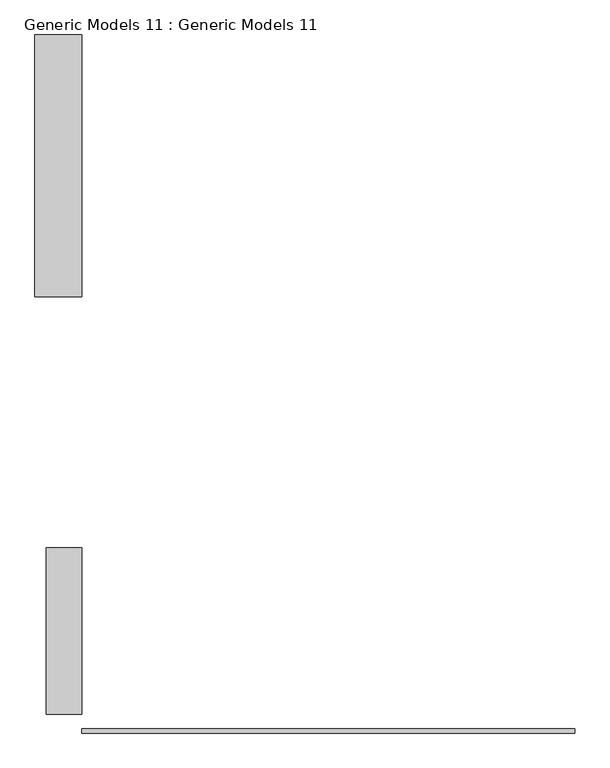
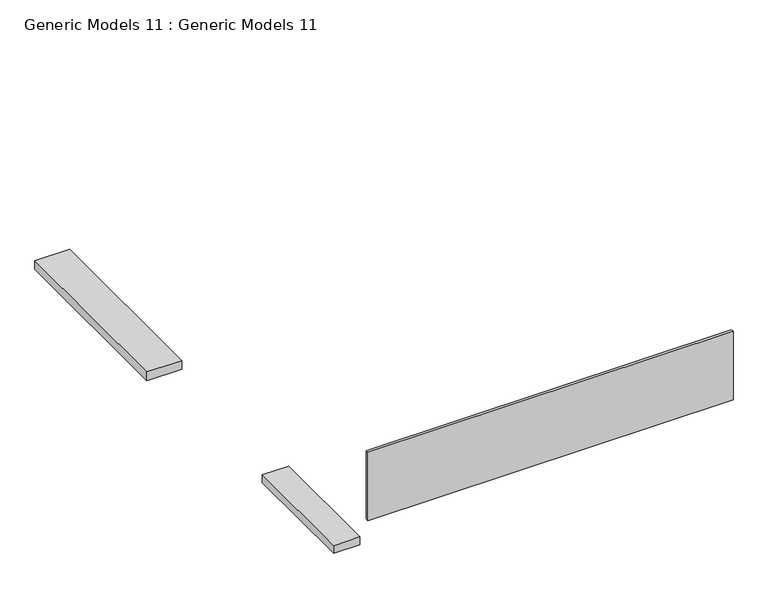
"""IFC4 building model written with IfcOpenShell, lengths in millimetres: proxy geometry, Generic Models 11 : Generic Models 11."""

from ifc_helpers import new_model, si_unit, frame, origin, place, context, project, spatial, polyline, outline, extrude, source, transform, mapped, element, save


def generic_models_11_generic_models_11_9e8de572(model_context):
    return source(origin(), model_context, "Body", "SweptSolid", [
        extrude(outline(polyline([(-11053.0120831, -12189.4945627), (-20044.6120831, -12189.4945627), (-20044.6120831, -12113.2945627), (-11053.0120831, -12113.2945627), (-11053.0120831, -12189.4945627)])), frame((0.0, 0.0, 6400.8), z_axis=(0.0, 0.0, 1.0), x_axis=(1.0, 0.0, 0.0)), (0.0, 0.0, 1.0), 1777.9376743),
        extrude(outline(polyline([(-20896.4433214, 534.8334881), (-20044.6120831, 534.8334881), (-20044.6120831, -4241.1507926), (-20896.4433214, -4241.1507926), (-20896.4433214, 534.8334881)])), frame((0.0, 0.0, 5519.0574769), z_axis=(0.0, 0.0, 1.0), x_axis=(1.0, 0.0, 0.0)), (0.0, 0.0, 1.0), 228.6),
        extrude(outline(polyline([(-20692.3120831, -8811.3488855), (-20044.6120831, -8811.3488855), (-20044.6120831, -11846.5945627), (-20692.3120831, -11846.5945627), (-20692.3120831, -8811.3488855)])), frame((0.0, 0.0, 5567.4357586), z_axis=(0.0, 0.0, 1.0), x_axis=(1.0, 0.0, 0.0)), (0.0, 0.0, 1.0), 203.2),
    ])


if __name__ == "__main__":
    model = new_model("IFC4")
    model_context = context("Model", 3, world=origin())
    ifc_project = project(units=[si_unit("LENGTHUNIT", "METRE", prefix="MILLI")], contexts=[model_context])
    site = spatial("IfcSite", under=ifc_project)
    building = spatial("IfcBuilding", under=site)
    placement = place(None, origin())
    generic_models_11_generic_models_11_shape = generic_models_11_generic_models_11_9e8de572(model_context)
    element("IfcBuildingElementProxy", 1, Name="Generic Models 11 : Generic Models 11", ObjectType="Generic Models 11 : Generic Models 11", at=placement, inside=building, context=model_context, shape_type="MappedRepresentation", body=[
        mapped(generic_models_11_generic_models_11_shape, transform((0.0, 0.0, 0.0), x_axis=(1.0, 0.0, 0.0), y_axis=(0.0, 1.0, 0.0), z_axis=(0.0, 0.0, 1.0))),
    ])
    save(model, "model.ifc")
